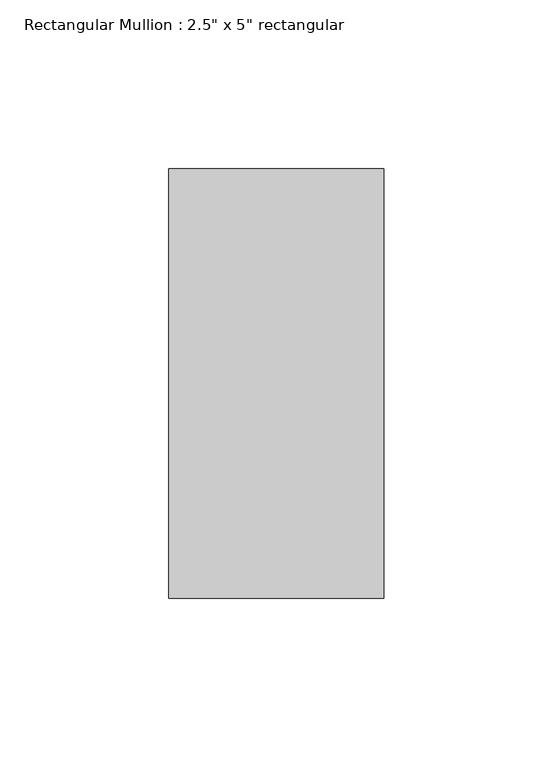
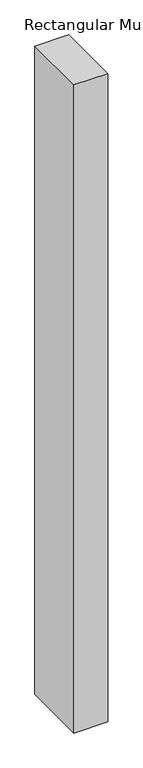
"""IFC4 building model written with IfcOpenShell, lengths in millimetres: member geometry."""

from ifc_helpers import new_model, si_unit, frame, origin, place, context, project, spatial, polyline, outline, extrude, source, transform, mapped, element, save


def member_c15214c4(model_context):
    return source(origin(), model_context, "Body", "SweptSolid", [
        extrude(outline(polyline([(0.0, 63.5), (0.0, -63.5), (-63.5, -63.5), (-63.5, 63.5), (0.0, 63.5)])), frame((0.0, 0.0, -1285.6336034), z_axis=(0.0, 0.0, 1.0), x_axis=(1.0, 0.0, 0.0)), (0.0, 0.0, 1.0), 1285.6336034),
    ])


if __name__ == "__main__":
    model = new_model("IFC4")
    model_context = context("Model", 3, world=origin())
    ifc_project = project(units=[si_unit("LENGTHUNIT", "METRE", prefix="MILLI")], contexts=[model_context])
    site = spatial("IfcSite", under=ifc_project)
    building = spatial("IfcBuilding", under=site)
    placement = place(None, origin())
    member_shape = member_c15214c4(model_context)
    element("IfcMember", 1, ObjectType="Rectangular Mullion : 2.5\" x 5\" rectangular", at=placement, inside=building, context=model_context, shape_type="MappedRepresentation", body=[
        mapped(member_shape, transform((0.0, 0.0, 0.0), x_axis=(1.0, 0.0, 0.0), y_axis=(0.0, 1.0, 0.0), z_axis=(0.0, 0.0, 1.0))),
    ])
    save(model, "model.ifc")

# Revit data of these elements
# Type "Rectangular Mullion : 2.5\" x 5\" rectangular"
#   built-in parameter 1007304 = 0.416667 (stored number, unit not read)
#   built-in parameter 1007301 = 0.104167 (stored number, unit not read)
#   built-in parameter 1007300 = 0.104167 (stored number, unit not read)
# Element 1 (IfcMember, "Rectangular Mullion : 2.5\" x 5\" rectangular")
#   Materials on its faces: "Aluminum"
# Materials
#   "Aluminum": class "Metal", colour RGB 247 247 247, transparency 0, Description = "Aluminum 6061", Cost = 0
